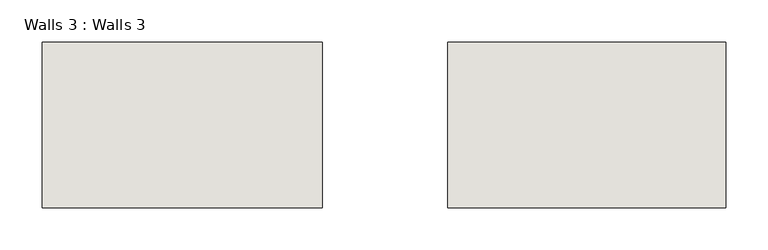
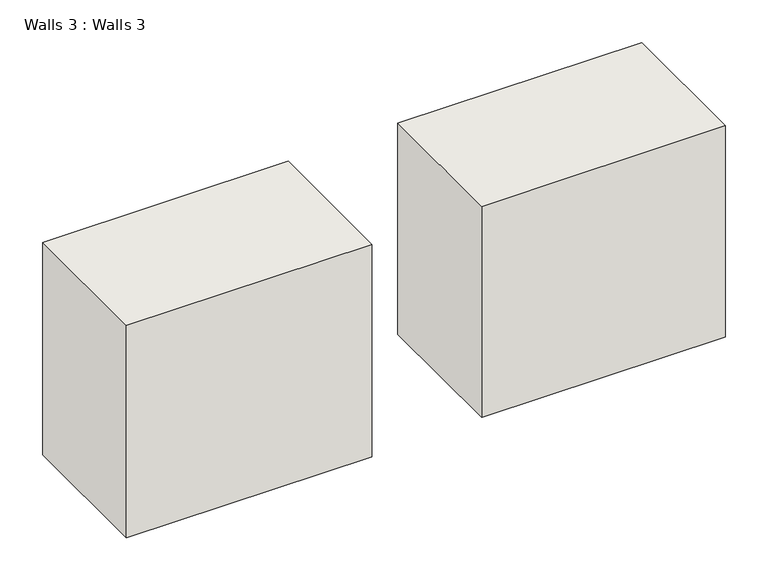
"""IFC4 building model written with IfcOpenShell, lengths in millimetres: wall geometry, Walls 3 : Walls 3."""

from ifc_helpers import new_model, si_unit, frame, origin, place, context, project, spatial, polyline, outline, extrude, source, transform, mapped, element, save


def walls_3_walls_3_68a7d47a(model_context):
    return source(origin(), model_context, "Body", "SweptSolid", [
        extrude(outline(polyline([(-2299.0046528, -3896.6207646), (-2630.349887, -3896.6207646), (-2630.349887, -3701.0259649), (-2299.0046528, -3701.0259649), (-2299.0046528, -3896.6207646)])), frame((0.0, 0.0, 7950.1039277), z_axis=(0.0, 0.0, 1.0), x_axis=(1.0, 0.0, 0.0)), (0.0, 0.0, 1.0), 303.601159),
        extrude(outline(polyline([(-1821.4270671, -3896.6207646), (-2150.604838, -3896.6207646), (-2150.604838, -3701.0259649), (-1821.4270671, -3701.0259649), (-1821.4270671, -3896.6207646)])), frame((0.0, 0.0, 7954.140465), z_axis=(0.0, 0.0, 1.0), x_axis=(1.0, 0.0, 0.0)), (0.0, 0.0, 1.0), 301.8885094),
    ])


if __name__ == "__main__":
    model = new_model("IFC4")
    model_context = context("Model", 3, world=origin())
    ifc_project = project(units=[si_unit("LENGTHUNIT", "METRE", prefix="MILLI")], contexts=[model_context])
    site = spatial("IfcSite", under=ifc_project)
    building = spatial("IfcBuilding", under=site)
    placement = place(None, origin())
    walls_3_walls_3_shape = walls_3_walls_3_68a7d47a(model_context)
    element("IfcWall", 1, ObjectType="Walls 3 : Walls 3", at=placement, inside=building, context=model_context, shape_type="MappedRepresentation", body=[
        mapped(walls_3_walls_3_shape, transform((0.0, 0.0, 0.0), x_axis=(1.0, 0.0, 0.0), y_axis=(0.0, 1.0, 0.0), z_axis=(0.0, 0.0, 1.0))),
    ])
    save(model, "model.ifc")

# Revit data of these elements
# Element 1 (IfcWall, "Walls 3 : Walls 3")
#   Materials on its faces: "Default Wall"
# Materials
#   "Default Wall": colour RGB 128 128 128, transparency 0
